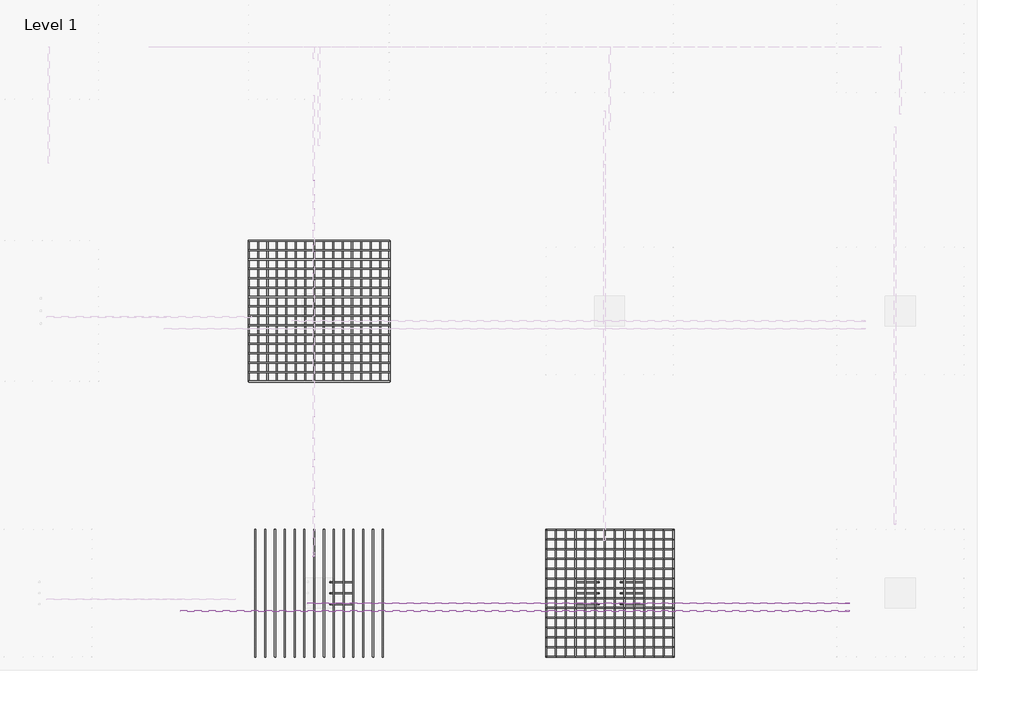
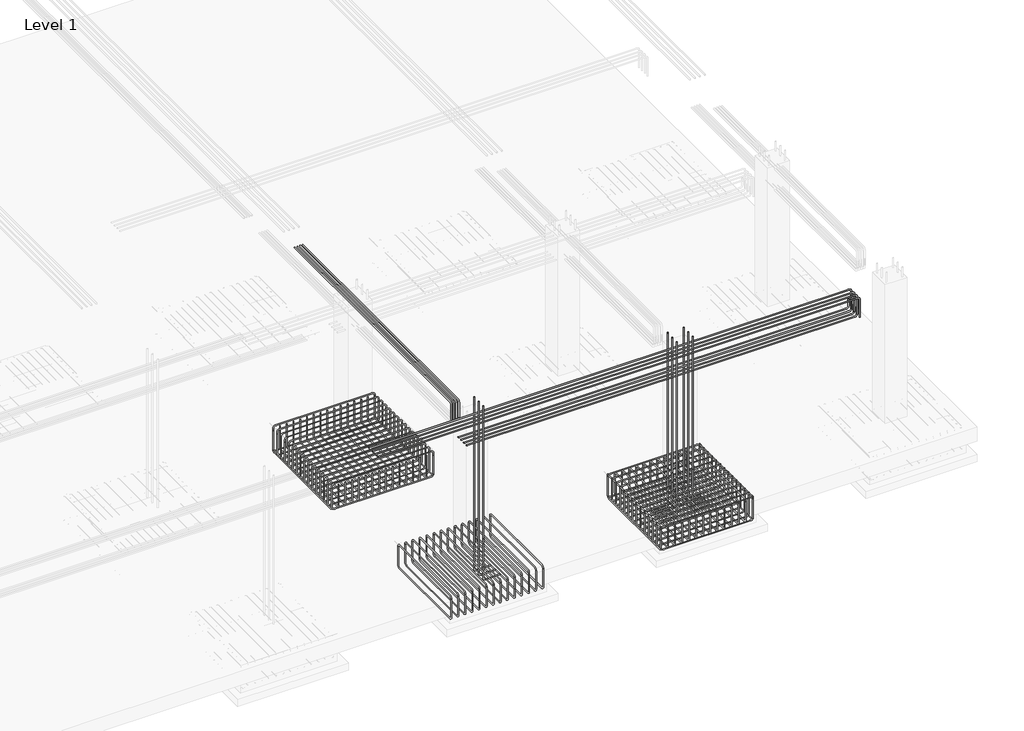
# One storey, part 6 of 17: 18 reinforcing bars.
"""IFC4 building model written with IfcOpenShell, lengths in millimetres."""

from ifc_helpers import new_model, si_unit, point, frame, origin, place, context, project, spatial, polyline, circle_curve, trimmed, segment, composite_curve, source, transform, mapped, element, save
from ifc_brep_helpers import swept_disk

model = new_model("IFC4")

# Units and contexts
model_context = context("Model", 3, world=origin())
ifc_project = project(units=[si_unit("LENGTHUNIT", "METRE", prefix="MILLI")], contexts=[model_context])

# Site, building, storey
site = spatial("IfcSite", under=ifc_project)
building = spatial("IfcBuilding", under=site)
storey = spatial("IfcBuildingStorey", under=building, Name="Level 1", Elevation=0.0)

# Reinforcing bars
placement = place(None, origin())
reinforcing_bar_shape = source(origin(), model_context, "Body", "SolidModel", [
    swept_disk(composite_curve([segment(polyline([(1252.6367997, -3580.990543, -96.0), (1252.6367997, -3580.990543, -504.0)]), True, "CONTINUOUS"), segment(trimmed(circle_curve(frame((1252.6367997, -3628.990543, -504.0), z_axis=(-1.0, 0.0, 0.0), x_axis=(0.0, 48.0, 0.0)), 48.0), [point((1252.6367997, -3580.990543, -504.0))], [point((1252.6367997, -3628.990543, -552.0))], True, "CARTESIAN"), True, "CONTINUOUS"), segment(polyline([(1252.6367997, -3628.990543, -552.0), (1252.6367997, -5436.990543, -552.0)]), True, "CONTINUOUS"), segment(trimmed(circle_curve(frame((1252.6367997, -5436.990543, -504.0), z_axis=(-1.0, 0.0, 0.0), x_axis=(0.0, 0.0, -48.0)), 48.0), [point((1252.6367997, -5436.990543, -552.0))], [point((1252.6367997, -5484.990543, -504.0))], True, "CARTESIAN"), True, "CONTINUOUS"), segment(polyline([(1252.6367997, -5484.990543, -504.0), (1252.6367997, -5484.990543, -96.0)]), True, "CONTINUOUS")], self_intersect=False), 8.0),
])
element("IfcReinforcingBar", 1, at=placement, inside=storey, context=model_context, shape_type="MappedRepresentation", body=[
    mapped(reinforcing_bar_shape, transform((0.0, 0.0, 0.0), x_axis=(1.0, 0.0, 0.0), y_axis=(0.0, 1.0, 0.0), z_axis=(0.0, 0.0, 1.0))),
    mapped(reinforcing_bar_shape, transform((-146.4615385, 0.0, 0.0), x_axis=(1.0, 0.0, 0.0), y_axis=(0.0, 1.0, 0.0), z_axis=(0.0, 0.0, 1.0))),
    mapped(reinforcing_bar_shape, transform((-292.9230769, 0.0, 0.0), x_axis=(1.0, 0.0, 0.0), y_axis=(0.0, 1.0, 0.0), z_axis=(0.0, 0.0, 1.0))),
    mapped(reinforcing_bar_shape, transform((-439.3846154, 0.0, 0.0), x_axis=(1.0, 0.0, 0.0), y_axis=(0.0, 1.0, 0.0), z_axis=(0.0, 0.0, 1.0))),
    mapped(reinforcing_bar_shape, transform((-585.8461538, 0.0, 0.0), x_axis=(1.0, 0.0, 0.0), y_axis=(0.0, 1.0, 0.0), z_axis=(0.0, 0.0, 1.0))),
    mapped(reinforcing_bar_shape, transform((-732.3076923, 0.0, 0.0), x_axis=(1.0, 0.0, 0.0), y_axis=(0.0, 1.0, 0.0), z_axis=(0.0, 0.0, 1.0))),
    mapped(reinforcing_bar_shape, transform((-878.7692308, 0.0, 0.0), x_axis=(1.0, 0.0, 0.0), y_axis=(0.0, 1.0, 0.0), z_axis=(0.0, 0.0, 1.0))),
    mapped(reinforcing_bar_shape, transform((-1025.2307692, 0.0, 0.0), x_axis=(1.0, 0.0, 0.0), y_axis=(0.0, 1.0, 0.0), z_axis=(0.0, 0.0, 1.0))),
    mapped(reinforcing_bar_shape, transform((-1171.6923077, 0.0, 0.0), x_axis=(1.0, 0.0, 0.0), y_axis=(0.0, 1.0, 0.0), z_axis=(0.0, 0.0, 1.0))),
    mapped(reinforcing_bar_shape, transform((-1318.1538462, 0.0, 0.0), x_axis=(1.0, 0.0, 0.0), y_axis=(0.0, 1.0, 0.0), z_axis=(0.0, 0.0, 1.0))),
    mapped(reinforcing_bar_shape, transform((-1464.6153846, 0.0, 0.0), x_axis=(1.0, 0.0, 0.0), y_axis=(0.0, 1.0, 0.0), z_axis=(0.0, 0.0, 1.0))),
    mapped(reinforcing_bar_shape, transform((-1611.0769231, 0.0, 0.0), x_axis=(1.0, 0.0, 0.0), y_axis=(0.0, 1.0, 0.0), z_axis=(0.0, 0.0, 1.0))),
    mapped(reinforcing_bar_shape, transform((-1757.5384615, 0.0, 0.0), x_axis=(1.0, 0.0, 0.0), y_axis=(0.0, 1.0, 0.0), z_axis=(0.0, 0.0, 1.0))),
    mapped(reinforcing_bar_shape, transform((-1904.0, 0.0, 0.0), x_axis=(1.0, 0.0, 0.0), y_axis=(0.0, 1.0, 0.0), z_axis=(0.0, 0.0, 1.0))),
])
reinforcing_bar_2_shape = source(origin(), model_context, "Body", "SolidModel", [
    swept_disk(composite_curve([segment(polyline([(-651.3632003, -3580.990543, -504.0), (-651.3632003, -3580.990543, -96.0)]), True, "CONTINUOUS"), segment(trimmed(circle_curve(frame((-651.3632003, -3628.990543, -96.0), z_axis=(1.0, 0.0, 0.0), x_axis=(0.0, 48.0, 0.0)), 48.0), [point((-651.3632003, -3580.990543, -96.0))], [point((-651.3632003, -3628.990543, -48.0))], True, "CARTESIAN"), True, "CONTINUOUS"), segment(polyline([(-651.3632003, -3628.990543, -48.0), (-651.3632003, -5436.990543, -48.0)]), True, "CONTINUOUS"), segment(trimmed(circle_curve(frame((-651.3632003, -5436.990543, -96.0), z_axis=(1.0, 0.0, 0.0), x_axis=(0.0, 0.0, 48.0)), 48.0), [point((-651.3632003, -5436.990543, -48.0))], [point((-651.3632003, -5484.990543, -96.0))], True, "CARTESIAN"), True, "CONTINUOUS"), segment(polyline([(-651.3632003, -5484.990543, -96.0), (-651.3632003, -5484.990543, -504.0)]), True, "CONTINUOUS")], self_intersect=False), 8.0),
])
element("IfcReinforcingBar", 2, at=placement, inside=storey, context=model_context, shape_type="MappedRepresentation", body=[
    mapped(reinforcing_bar_2_shape, transform((0.0, 0.0, 0.0), x_axis=(1.0, 0.0, 0.0), y_axis=(0.0, 1.0, 0.0), z_axis=(0.0, 0.0, 1.0))),
    mapped(reinforcing_bar_2_shape, transform((146.4615385, 0.0, 0.0), x_axis=(1.0, 0.0, 0.0), y_axis=(0.0, 1.0, 0.0), z_axis=(0.0, 0.0, 1.0))),
    mapped(reinforcing_bar_2_shape, transform((292.9230769, 0.0, 0.0), x_axis=(1.0, 0.0, 0.0), y_axis=(0.0, 1.0, 0.0), z_axis=(0.0, 0.0, 1.0))),
    mapped(reinforcing_bar_2_shape, transform((439.3846154, 0.0, 0.0), x_axis=(1.0, 0.0, 0.0), y_axis=(0.0, 1.0, 0.0), z_axis=(0.0, 0.0, 1.0))),
    mapped(reinforcing_bar_2_shape, transform((585.8461538, 0.0, 0.0), x_axis=(1.0, 0.0, 0.0), y_axis=(0.0, 1.0, 0.0), z_axis=(0.0, 0.0, 1.0))),
    mapped(reinforcing_bar_2_shape, transform((732.3076923, 0.0, 0.0), x_axis=(1.0, 0.0, 0.0), y_axis=(0.0, 1.0, 0.0), z_axis=(0.0, 0.0, 1.0))),
    mapped(reinforcing_bar_2_shape, transform((878.7692308, 0.0, 0.0), x_axis=(1.0, 0.0, 0.0), y_axis=(0.0, 1.0, 0.0), z_axis=(0.0, 0.0, 1.0))),
    mapped(reinforcing_bar_2_shape, transform((1025.2307692, 0.0, 0.0), x_axis=(1.0, 0.0, 0.0), y_axis=(0.0, 1.0, 0.0), z_axis=(0.0, 0.0, 1.0))),
    mapped(reinforcing_bar_2_shape, transform((1171.6923077, 0.0, 0.0), x_axis=(1.0, 0.0, 0.0), y_axis=(0.0, 1.0, 0.0), z_axis=(0.0, 0.0, 1.0))),
    mapped(reinforcing_bar_2_shape, transform((1318.1538462, 0.0, 0.0), x_axis=(1.0, 0.0, 0.0), y_axis=(0.0, 1.0, 0.0), z_axis=(0.0, 0.0, 1.0))),
    mapped(reinforcing_bar_2_shape, transform((1464.6153846, 0.0, 0.0), x_axis=(1.0, 0.0, 0.0), y_axis=(0.0, 1.0, 0.0), z_axis=(0.0, 0.0, 1.0))),
    mapped(reinforcing_bar_2_shape, transform((1611.0769231, 0.0, 0.0), x_axis=(1.0, 0.0, 0.0), y_axis=(0.0, 1.0, 0.0), z_axis=(0.0, 0.0, 1.0))),
    mapped(reinforcing_bar_2_shape, transform((1757.5384615, 0.0, 0.0), x_axis=(1.0, 0.0, 0.0), y_axis=(0.0, 1.0, 0.0), z_axis=(0.0, 0.0, 1.0))),
    mapped(reinforcing_bar_2_shape, transform((1904.0, 0.0, 0.0), x_axis=(1.0, 0.0, 0.0), y_axis=(0.0, 1.0, 0.0), z_axis=(0.0, 0.0, 1.0))),
])
reinforcing_bar_3_shape = source(origin(), model_context, "Body", "SolidModel", [
    swept_disk(composite_curve([segment(polyline([(813.2521843, -4698.490543, -550.0), (516.1367997, -4698.490543, -550.0)]), True, "CONTINUOUS"), segment(trimmed(circle_curve(frame((516.1367997, -4698.490543, -500.0), z_axis=(0.0, 1.0, 0.0), x_axis=(0.0, 0.0, -50.0)), 50.0), [point((516.1367997, -4698.490543, -550.0))], [point((466.1367997, -4698.490543, -500.0))], True, "CARTESIAN"), True, "CONTINUOUS"), segment(polyline([(466.1367997, -4698.490543, -500.0), (466.1367997, -4698.490543, 3260.0)]), True, "CONTINUOUS")], self_intersect=False), 10.0),
])
element("IfcReinforcingBar", 3, at=placement, inside=storey, context=model_context, shape_type="MappedRepresentation", body=[
    mapped(reinforcing_bar_3_shape, transform((0.0, 0.0, 0.0), x_axis=(1.0, 0.0, 0.0), y_axis=(0.0, 1.0, 0.0), z_axis=(0.0, 0.0, 1.0))),
    mapped(reinforcing_bar_3_shape, transform((0.0, 165.5, 0.0), x_axis=(1.0, 0.0, 0.0), y_axis=(0.0, 1.0, 0.0), z_axis=(0.0, 0.0, 1.0))),
    mapped(reinforcing_bar_3_shape, transform((0.0, 331.0, 0.0), x_axis=(1.0, 0.0, 0.0), y_axis=(0.0, 1.0, 0.0), z_axis=(0.0, 0.0, 1.0))),
])
reinforcing_bar_4_shape = source(origin(), model_context, "Body", "SolidModel", [
    swept_disk(composite_curve([segment(polyline([(3693.6367997, -3580.990543, -40.0), (3693.6367997, -3580.990543, -504.0)]), True, "CONTINUOUS"), segment(trimmed(circle_curve(frame((3741.6367997, -3580.990543, -504.0), z_axis=(0.0, -1.0, 0.0), x_axis=(-48.0, 0.0, 0.0)), 48.0), [point((3693.6367997, -3580.990543, -504.0))], [point((3741.6367997, -3580.990543, -552.0))], True, "CARTESIAN"), True, "CONTINUOUS"), segment(polyline([(3741.6367997, -3580.990543, -552.0), (5549.6367997, -3580.990543, -552.0)]), True, "CONTINUOUS"), segment(trimmed(circle_curve(frame((5549.6367997, -3580.990543, -504.0), z_axis=(0.0, -1.0, 0.0), x_axis=(0.0, 0.0, -48.0)), 48.0), [point((5549.6367997, -3580.990543, -552.0))], [point((5597.6367997, -3580.990543, -504.0))], True, "CARTESIAN"), True, "CONTINUOUS"), segment(polyline([(5597.6367997, -3580.990543, -504.0), (5597.6367997, -3580.990543, -40.0)]), True, "CONTINUOUS")], self_intersect=False), 8.0),
])
element("IfcReinforcingBar", 4, at=placement, inside=storey, context=model_context, shape_type="MappedRepresentation", body=[
    mapped(reinforcing_bar_4_shape, transform((0.0, 0.0, 0.0), x_axis=(1.0, 0.0, 0.0), y_axis=(0.0, 1.0, 0.0), z_axis=(0.0, 0.0, 1.0))),
    mapped(reinforcing_bar_4_shape, transform((0.0, -146.4615385, 0.0), x_axis=(1.0, 0.0, 0.0), y_axis=(0.0, 1.0, 0.0), z_axis=(0.0, 0.0, 1.0))),
    mapped(reinforcing_bar_4_shape, transform((0.0, -292.9230769, 0.0), x_axis=(1.0, 0.0, 0.0), y_axis=(0.0, 1.0, 0.0), z_axis=(0.0, 0.0, 1.0))),
    mapped(reinforcing_bar_4_shape, transform((0.0, -439.3846154, 0.0), x_axis=(1.0, 0.0, 0.0), y_axis=(0.0, 1.0, 0.0), z_axis=(0.0, 0.0, 1.0))),
    mapped(reinforcing_bar_4_shape, transform((0.0, -585.8461538, 0.0), x_axis=(1.0, 0.0, 0.0), y_axis=(0.0, 1.0, 0.0), z_axis=(0.0, 0.0, 1.0))),
    mapped(reinforcing_bar_4_shape, transform((0.0, -732.3076923, 0.0), x_axis=(1.0, 0.0, 0.0), y_axis=(0.0, 1.0, 0.0), z_axis=(0.0, 0.0, 1.0))),
    mapped(reinforcing_bar_4_shape, transform((0.0, -878.7692308, 0.0), x_axis=(1.0, 0.0, 0.0), y_axis=(0.0, 1.0, 0.0), z_axis=(0.0, 0.0, 1.0))),
    mapped(reinforcing_bar_4_shape, transform((0.0, -1025.2307692, 0.0), x_axis=(1.0, 0.0, 0.0), y_axis=(0.0, 1.0, 0.0), z_axis=(0.0, 0.0, 1.0))),
    mapped(reinforcing_bar_4_shape, transform((0.0, -1171.6923077, 0.0), x_axis=(1.0, 0.0, 0.0), y_axis=(0.0, 1.0, 0.0), z_axis=(0.0, 0.0, 1.0))),
    mapped(reinforcing_bar_4_shape, transform((0.0, -1318.1538462, 0.0), x_axis=(1.0, 0.0, 0.0), y_axis=(0.0, 1.0, 0.0), z_axis=(0.0, 0.0, 1.0))),
    mapped(reinforcing_bar_4_shape, transform((0.0, -1464.6153846, 0.0), x_axis=(1.0, 0.0, 0.0), y_axis=(0.0, 1.0, 0.0), z_axis=(0.0, 0.0, 1.0))),
    mapped(reinforcing_bar_4_shape, transform((0.0, -1611.0769231, 0.0), x_axis=(1.0, 0.0, 0.0), y_axis=(0.0, 1.0, 0.0), z_axis=(0.0, 0.0, 1.0))),
    mapped(reinforcing_bar_4_shape, transform((0.0, -1757.5384615, 0.0), x_axis=(1.0, 0.0, 0.0), y_axis=(0.0, 1.0, 0.0), z_axis=(0.0, 0.0, 1.0))),
    mapped(reinforcing_bar_4_shape, transform((0.0, -1904.0, 0.0), x_axis=(1.0, 0.0, 0.0), y_axis=(0.0, 1.0, 0.0), z_axis=(0.0, 0.0, 1.0))),
])
reinforcing_bar_5_shape = source(origin(), model_context, "Body", "SolidModel", [
    swept_disk(composite_curve([segment(polyline([(3693.6367997, -5484.990543, -504.0), (3693.6367997, -5484.990543, -96.0)]), True, "CONTINUOUS"), segment(trimmed(circle_curve(frame((3741.6367997, -5484.990543, -96.0), z_axis=(0.0, 1.0, 0.0), x_axis=(-48.0, 0.0, 0.0)), 48.0), [point((3693.6367997, -5484.990543, -96.0))], [point((3741.6367997, -5484.990543, -48.0))], True, "CARTESIAN"), True, "CONTINUOUS"), segment(polyline([(3741.6367997, -5484.990543, -48.0), (5549.6367997, -5484.990543, -48.0)]), True, "CONTINUOUS"), segment(trimmed(circle_curve(frame((5549.6367997, -5484.990543, -96.0), z_axis=(0.0, 1.0, 0.0), x_axis=(0.0, 0.0, 48.0)), 48.0), [point((5549.6367997, -5484.990543, -48.0))], [point((5597.6367997, -5484.990543, -96.0))], True, "CARTESIAN"), True, "CONTINUOUS"), segment(polyline([(5597.6367997, -5484.990543, -96.0), (5597.6367997, -5484.990543, -504.0)]), True, "CONTINUOUS")], self_intersect=False), 8.0),
])
element("IfcReinforcingBar", 5, at=placement, inside=storey, context=model_context, shape_type="MappedRepresentation", body=[
    mapped(reinforcing_bar_5_shape, transform((0.0, 0.0, 0.0), x_axis=(1.0, 0.0, 0.0), y_axis=(0.0, 1.0, 0.0), z_axis=(0.0, 0.0, 1.0))),
    mapped(reinforcing_bar_5_shape, transform((0.0, 146.4615385, 0.0), x_axis=(1.0, 0.0, 0.0), y_axis=(0.0, 1.0, 0.0), z_axis=(0.0, 0.0, 1.0))),
    mapped(reinforcing_bar_5_shape, transform((0.0, 292.9230769, 0.0), x_axis=(1.0, 0.0, 0.0), y_axis=(0.0, 1.0, 0.0), z_axis=(0.0, 0.0, 1.0))),
    mapped(reinforcing_bar_5_shape, transform((0.0, 439.3846154, 0.0), x_axis=(1.0, 0.0, 0.0), y_axis=(0.0, 1.0, 0.0), z_axis=(0.0, 0.0, 1.0))),
    mapped(reinforcing_bar_5_shape, transform((0.0, 585.8461538, 0.0), x_axis=(1.0, 0.0, 0.0), y_axis=(0.0, 1.0, 0.0), z_axis=(0.0, 0.0, 1.0))),
    mapped(reinforcing_bar_5_shape, transform((0.0, 732.3076923, 0.0), x_axis=(1.0, 0.0, 0.0), y_axis=(0.0, 1.0, 0.0), z_axis=(0.0, 0.0, 1.0))),
    mapped(reinforcing_bar_5_shape, transform((0.0, 878.7692308, 0.0), x_axis=(1.0, 0.0, 0.0), y_axis=(0.0, 1.0, 0.0), z_axis=(0.0, 0.0, 1.0))),
    mapped(reinforcing_bar_5_shape, transform((0.0, 1025.2307692, 0.0), x_axis=(1.0, 0.0, 0.0), y_axis=(0.0, 1.0, 0.0), z_axis=(0.0, 0.0, 1.0))),
    mapped(reinforcing_bar_5_shape, transform((0.0, 1171.6923077, 0.0), x_axis=(1.0, 0.0, 0.0), y_axis=(0.0, 1.0, 0.0), z_axis=(0.0, 0.0, 1.0))),
    mapped(reinforcing_bar_5_shape, transform((0.0, 1318.1538462, 0.0), x_axis=(1.0, 0.0, 0.0), y_axis=(0.0, 1.0, 0.0), z_axis=(0.0, 0.0, 1.0))),
    mapped(reinforcing_bar_5_shape, transform((0.0, 1464.6153846, 0.0), x_axis=(1.0, 0.0, 0.0), y_axis=(0.0, 1.0, 0.0), z_axis=(0.0, 0.0, 1.0))),
    mapped(reinforcing_bar_5_shape, transform((0.0, 1611.0769231, 0.0), x_axis=(1.0, 0.0, 0.0), y_axis=(0.0, 1.0, 0.0), z_axis=(0.0, 0.0, 1.0))),
    mapped(reinforcing_bar_5_shape, transform((0.0, 1757.5384615, 0.0), x_axis=(1.0, 0.0, 0.0), y_axis=(0.0, 1.0, 0.0), z_axis=(0.0, 0.0, 1.0))),
    mapped(reinforcing_bar_5_shape, transform((0.0, 1904.0, 0.0), x_axis=(1.0, 0.0, 0.0), y_axis=(0.0, 1.0, 0.0), z_axis=(0.0, 0.0, 1.0))),
])
reinforcing_bar_6_shape = source(origin(), model_context, "Body", "SolidModel", [
    swept_disk(composite_curve([segment(polyline([(5597.6367997, -3580.990543, -96.0), (5597.6367997, -3580.990543, -504.0)]), True, "CONTINUOUS"), segment(trimmed(circle_curve(frame((5597.6367997, -3628.990543, -504.0), z_axis=(-1.0, 0.0, 0.0), x_axis=(0.0, 48.0, 0.0)), 48.0), [point((5597.6367997, -3580.990543, -504.0))], [point((5597.6367997, -3628.990543, -552.0))], True, "CARTESIAN"), True, "CONTINUOUS"), segment(polyline([(5597.6367997, -3628.990543, -552.0), (5597.6367997, -5436.990543, -552.0)]), True, "CONTINUOUS"), segment(trimmed(circle_curve(frame((5597.6367997, -5436.990543, -504.0), z_axis=(-1.0, 0.0, 0.0), x_axis=(0.0, 0.0, -48.0)), 48.0), [point((5597.6367997, -5436.990543, -552.0))], [point((5597.6367997, -5484.990543, -504.0))], True, "CARTESIAN"), True, "CONTINUOUS"), segment(polyline([(5597.6367997, -5484.990543, -504.0), (5597.6367997, -5484.990543, -96.0)]), True, "CONTINUOUS")], self_intersect=False), 8.0),
])
element("IfcReinforcingBar", 6, at=placement, inside=storey, context=model_context, shape_type="MappedRepresentation", body=[
    mapped(reinforcing_bar_6_shape, transform((0.0, 0.0, 0.0), x_axis=(1.0, 0.0, 0.0), y_axis=(0.0, 1.0, 0.0), z_axis=(0.0, 0.0, 1.0))),
    mapped(reinforcing_bar_6_shape, transform((-146.4615385, 0.0, 0.0), x_axis=(1.0, 0.0, 0.0), y_axis=(0.0, 1.0, 0.0), z_axis=(0.0, 0.0, 1.0))),
    mapped(reinforcing_bar_6_shape, transform((-292.9230769, 0.0, 0.0), x_axis=(1.0, 0.0, 0.0), y_axis=(0.0, 1.0, 0.0), z_axis=(0.0, 0.0, 1.0))),
    mapped(reinforcing_bar_6_shape, transform((-439.3846154, 0.0, 0.0), x_axis=(1.0, 0.0, 0.0), y_axis=(0.0, 1.0, 0.0), z_axis=(0.0, 0.0, 1.0))),
    mapped(reinforcing_bar_6_shape, transform((-585.8461538, 0.0, 0.0), x_axis=(1.0, 0.0, 0.0), y_axis=(0.0, 1.0, 0.0), z_axis=(0.0, 0.0, 1.0))),
    mapped(reinforcing_bar_6_shape, transform((-732.3076923, 0.0, 0.0), x_axis=(1.0, 0.0, 0.0), y_axis=(0.0, 1.0, 0.0), z_axis=(0.0, 0.0, 1.0))),
    mapped(reinforcing_bar_6_shape, transform((-878.7692308, 0.0, 0.0), x_axis=(1.0, 0.0, 0.0), y_axis=(0.0, 1.0, 0.0), z_axis=(0.0, 0.0, 1.0))),
    mapped(reinforcing_bar_6_shape, transform((-1025.2307692, 0.0, 0.0), x_axis=(1.0, 0.0, 0.0), y_axis=(0.0, 1.0, 0.0), z_axis=(0.0, 0.0, 1.0))),
    mapped(reinforcing_bar_6_shape, transform((-1171.6923077, 0.0, 0.0), x_axis=(1.0, 0.0, 0.0), y_axis=(0.0, 1.0, 0.0), z_axis=(0.0, 0.0, 1.0))),
    mapped(reinforcing_bar_6_shape, transform((-1318.1538462, 0.0, 0.0), x_axis=(1.0, 0.0, 0.0), y_axis=(0.0, 1.0, 0.0), z_axis=(0.0, 0.0, 1.0))),
    mapped(reinforcing_bar_6_shape, transform((-1464.6153846, 0.0, 0.0), x_axis=(1.0, 0.0, 0.0), y_axis=(0.0, 1.0, 0.0), z_axis=(0.0, 0.0, 1.0))),
    mapped(reinforcing_bar_6_shape, transform((-1611.0769231, 0.0, 0.0), x_axis=(1.0, 0.0, 0.0), y_axis=(0.0, 1.0, 0.0), z_axis=(0.0, 0.0, 1.0))),
    mapped(reinforcing_bar_6_shape, transform((-1757.5384615, 0.0, 0.0), x_axis=(1.0, 0.0, 0.0), y_axis=(0.0, 1.0, 0.0), z_axis=(0.0, 0.0, 1.0))),
    mapped(reinforcing_bar_6_shape, transform((-1904.0, 0.0, 0.0), x_axis=(1.0, 0.0, 0.0), y_axis=(0.0, 1.0, 0.0), z_axis=(0.0, 0.0, 1.0))),
])
reinforcing_bar_7_shape = source(origin(), model_context, "Body", "SolidModel", [
    swept_disk(composite_curve([segment(polyline([(3693.6367997, -3580.990543, -504.0), (3693.6367997, -3580.990543, -96.0)]), True, "CONTINUOUS"), segment(trimmed(circle_curve(frame((3693.6367997, -3628.990543, -96.0), z_axis=(1.0, 0.0, 0.0), x_axis=(0.0, 48.0, 0.0)), 48.0), [point((3693.6367997, -3580.990543, -96.0))], [point((3693.6367997, -3628.990543, -48.0))], True, "CARTESIAN"), True, "CONTINUOUS"), segment(polyline([(3693.6367997, -3628.990543, -48.0), (3693.6367997, -5436.990543, -48.0)]), True, "CONTINUOUS"), segment(trimmed(circle_curve(frame((3693.6367997, -5436.990543, -96.0), z_axis=(1.0, 0.0, 0.0), x_axis=(0.0, 0.0, 48.0)), 48.0), [point((3693.6367997, -5436.990543, -48.0))], [point((3693.6367997, -5484.990543, -96.0))], True, "CARTESIAN"), True, "CONTINUOUS"), segment(polyline([(3693.6367997, -5484.990543, -96.0), (3693.6367997, -5484.990543, -504.0)]), True, "CONTINUOUS")], self_intersect=False), 8.0),
])
element("IfcReinforcingBar", 7, at=placement, inside=storey, context=model_context, shape_type="MappedRepresentation", body=[
    mapped(reinforcing_bar_7_shape, transform((0.0, 0.0, 0.0), x_axis=(1.0, 0.0, 0.0), y_axis=(0.0, 1.0, 0.0), z_axis=(0.0, 0.0, 1.0))),
    mapped(reinforcing_bar_7_shape, transform((146.4615385, 0.0, 0.0), x_axis=(1.0, 0.0, 0.0), y_axis=(0.0, 1.0, 0.0), z_axis=(0.0, 0.0, 1.0))),
    mapped(reinforcing_bar_7_shape, transform((292.9230769, 0.0, 0.0), x_axis=(1.0, 0.0, 0.0), y_axis=(0.0, 1.0, 0.0), z_axis=(0.0, 0.0, 1.0))),
    mapped(reinforcing_bar_7_shape, transform((439.3846154, 0.0, 0.0), x_axis=(1.0, 0.0, 0.0), y_axis=(0.0, 1.0, 0.0), z_axis=(0.0, 0.0, 1.0))),
    mapped(reinforcing_bar_7_shape, transform((585.8461538, 0.0, 0.0), x_axis=(1.0, 0.0, 0.0), y_axis=(0.0, 1.0, 0.0), z_axis=(0.0, 0.0, 1.0))),
    mapped(reinforcing_bar_7_shape, transform((732.3076923, 0.0, 0.0), x_axis=(1.0, 0.0, 0.0), y_axis=(0.0, 1.0, 0.0), z_axis=(0.0, 0.0, 1.0))),
    mapped(reinforcing_bar_7_shape, transform((878.7692308, 0.0, 0.0), x_axis=(1.0, 0.0, 0.0), y_axis=(0.0, 1.0, 0.0), z_axis=(0.0, 0.0, 1.0))),
    mapped(reinforcing_bar_7_shape, transform((1025.2307692, 0.0, 0.0), x_axis=(1.0, 0.0, 0.0), y_axis=(0.0, 1.0, 0.0), z_axis=(0.0, 0.0, 1.0))),
    mapped(reinforcing_bar_7_shape, transform((1171.6923077, 0.0, 0.0), x_axis=(1.0, 0.0, 0.0), y_axis=(0.0, 1.0, 0.0), z_axis=(0.0, 0.0, 1.0))),
    mapped(reinforcing_bar_7_shape, transform((1318.1538462, 0.0, 0.0), x_axis=(1.0, 0.0, 0.0), y_axis=(0.0, 1.0, 0.0), z_axis=(0.0, 0.0, 1.0))),
    mapped(reinforcing_bar_7_shape, transform((1464.6153846, 0.0, 0.0), x_axis=(1.0, 0.0, 0.0), y_axis=(0.0, 1.0, 0.0), z_axis=(0.0, 0.0, 1.0))),
    mapped(reinforcing_bar_7_shape, transform((1611.0769231, 0.0, 0.0), x_axis=(1.0, 0.0, 0.0), y_axis=(0.0, 1.0, 0.0), z_axis=(0.0, 0.0, 1.0))),
    mapped(reinforcing_bar_7_shape, transform((1757.5384615, 0.0, 0.0), x_axis=(1.0, 0.0, 0.0), y_axis=(0.0, 1.0, 0.0), z_axis=(0.0, 0.0, 1.0))),
    mapped(reinforcing_bar_7_shape, transform((1904.0, 0.0, 0.0), x_axis=(1.0, 0.0, 0.0), y_axis=(0.0, 1.0, 0.0), z_axis=(0.0, 0.0, 1.0))),
])
reinforcing_bar_8_shape = source(origin(), model_context, "Body", "SolidModel", [
    swept_disk(composite_curve([segment(polyline([(4133.0214151, -4367.490543, -550.0), (4430.1367997, -4367.490543, -550.0)]), True, "CONTINUOUS"), segment(trimmed(circle_curve(frame((4430.1367997, -4367.490543, -500.0), z_axis=(0.0, -1.0, 0.0), x_axis=(0.0, 0.0, -50.0)), 50.0), [point((4430.1367997, -4367.490543, -550.0))], [point((4480.1367997, -4367.490543, -500.0))], True, "CARTESIAN"), True, "CONTINUOUS"), segment(polyline([(4480.1367997, -4367.490543, -500.0), (4480.1367997, -4367.490543, 3260.0)]), True, "CONTINUOUS")], self_intersect=False), 10.0),
])
element("IfcReinforcingBar", 8, at=placement, inside=storey, context=model_context, shape_type="MappedRepresentation", body=[
    mapped(reinforcing_bar_8_shape, transform((0.0, 0.0, 0.0), x_axis=(1.0, 0.0, 0.0), y_axis=(0.0, 1.0, 0.0), z_axis=(0.0, 0.0, 1.0))),
    mapped(reinforcing_bar_8_shape, transform((0.0, -165.5, 0.0), x_axis=(1.0, 0.0, 0.0), y_axis=(0.0, 1.0, 0.0), z_axis=(0.0, 0.0, 1.0))),
    mapped(reinforcing_bar_8_shape, transform((0.0, -331.0, 0.0), x_axis=(1.0, 0.0, 0.0), y_axis=(0.0, 1.0, 0.0), z_axis=(0.0, 0.0, 1.0))),
])
reinforcing_bar_9_shape = source(origin(), model_context, "Body", "SolidModel", [
    swept_disk(composite_curve([segment(polyline([(5158.2521843, -4698.490543, -550.0), (4861.1367997, -4698.490543, -550.0)]), True, "CONTINUOUS"), segment(trimmed(circle_curve(frame((4861.1367997, -4698.490543, -500.0), z_axis=(0.0, 1.0, 0.0), x_axis=(0.0, 0.0, -50.0)), 50.0), [point((4861.1367997, -4698.490543, -550.0))], [point((4811.1367997, -4698.490543, -500.0))], True, "CARTESIAN"), True, "CONTINUOUS"), segment(polyline([(4811.1367997, -4698.490543, -500.0), (4811.1367997, -4698.490543, 3260.0)]), True, "CONTINUOUS")], self_intersect=False), 10.0),
])
element("IfcReinforcingBar", 9, at=placement, inside=storey, context=model_context, shape_type="MappedRepresentation", body=[
    mapped(reinforcing_bar_9_shape, transform((0.0, 0.0, 0.0), x_axis=(1.0, 0.0, 0.0), y_axis=(0.0, 1.0, 0.0), z_axis=(0.0, 0.0, 1.0))),
    mapped(reinforcing_bar_9_shape, transform((0.0, 165.5, 0.0), x_axis=(1.0, 0.0, 0.0), y_axis=(0.0, 1.0, 0.0), z_axis=(0.0, 0.0, 1.0))),
    mapped(reinforcing_bar_9_shape, transform((0.0, 331.0, 0.0), x_axis=(1.0, 0.0, 0.0), y_axis=(0.0, 1.0, 0.0), z_axis=(0.0, 0.0, 1.0))),
])
reinforcing_bar_10_shape = source(origin(), model_context, "Body", "SolidModel", [
    swept_disk(composite_curve([segment(polyline([(-751.3632003, 736.009457, -140.0), (-751.3632003, 736.009457, -554.0)]), True, "CONTINUOUS"), segment(trimmed(circle_curve(frame((-703.3632003, 736.009457, -554.0), z_axis=(0.0, -1.0, 0.0), x_axis=(-48.0, 0.0, 0.0)), 48.0), [point((-751.3632003, 736.009457, -554.0))], [point((-703.3632003, 736.009457, -602.0))], True, "CARTESIAN"), True, "CONTINUOUS"), segment(polyline([(-703.3632003, 736.009457, -602.0), (1304.6367997, 736.009457, -602.0)]), True, "CONTINUOUS"), segment(trimmed(circle_curve(frame((1304.6367997, 736.009457, -554.0), z_axis=(0.0, -1.0, 0.0), x_axis=(0.0, 0.0, -48.0)), 48.0), [point((1304.6367997, 736.009457, -602.0))], [point((1352.6367997, 736.009457, -554.0))], True, "CARTESIAN"), True, "CONTINUOUS"), segment(polyline([(1352.6367997, 736.009457, -554.0), (1352.6367997, 736.009457, -140.0)]), True, "CONTINUOUS")], self_intersect=False), 8.0),
])
element("IfcReinforcingBar", 10, at=placement, inside=storey, context=model_context, shape_type="MappedRepresentation", body=[
    mapped(reinforcing_bar_10_shape, transform((0.0, 0.0, 0.0), x_axis=(1.0, 0.0, 0.0), y_axis=(0.0, 1.0, 0.0), z_axis=(0.0, 0.0, 1.0))),
    mapped(reinforcing_bar_10_shape, transform((0.0, -140.2666667, 0.0), x_axis=(1.0, 0.0, 0.0), y_axis=(0.0, 1.0, 0.0), z_axis=(0.0, 0.0, 1.0))),
    mapped(reinforcing_bar_10_shape, transform((0.0, -280.5333333, 0.0), x_axis=(1.0, 0.0, 0.0), y_axis=(0.0, 1.0, 0.0), z_axis=(0.0, 0.0, 1.0))),
    mapped(reinforcing_bar_10_shape, transform((0.0, -420.8, 0.0), x_axis=(1.0, 0.0, 0.0), y_axis=(0.0, 1.0, 0.0), z_axis=(0.0, 0.0, 1.0))),
    mapped(reinforcing_bar_10_shape, transform((0.0, -561.0666667, 0.0), x_axis=(1.0, 0.0, 0.0), y_axis=(0.0, 1.0, 0.0), z_axis=(0.0, 0.0, 1.0))),
    mapped(reinforcing_bar_10_shape, transform((0.0, -701.3333333, 0.0), x_axis=(1.0, 0.0, 0.0), y_axis=(0.0, 1.0, 0.0), z_axis=(0.0, 0.0, 1.0))),
    mapped(reinforcing_bar_10_shape, transform((0.0, -841.6, 0.0), x_axis=(1.0, 0.0, 0.0), y_axis=(0.0, 1.0, 0.0), z_axis=(0.0, 0.0, 1.0))),
    mapped(reinforcing_bar_10_shape, transform((0.0, -981.8666667, 0.0), x_axis=(1.0, 0.0, 0.0), y_axis=(0.0, 1.0, 0.0), z_axis=(0.0, 0.0, 1.0))),
    mapped(reinforcing_bar_10_shape, transform((0.0, -1122.1333333, 0.0), x_axis=(1.0, 0.0, 0.0), y_axis=(0.0, 1.0, 0.0), z_axis=(0.0, 0.0, 1.0))),
    mapped(reinforcing_bar_10_shape, transform((0.0, -1262.4, 0.0), x_axis=(1.0, 0.0, 0.0), y_axis=(0.0, 1.0, 0.0), z_axis=(0.0, 0.0, 1.0))),
    mapped(reinforcing_bar_10_shape, transform((0.0, -1402.6666667, 0.0), x_axis=(1.0, 0.0, 0.0), y_axis=(0.0, 1.0, 0.0), z_axis=(0.0, 0.0, 1.0))),
    mapped(reinforcing_bar_10_shape, transform((0.0, -1542.9333333, 0.0), x_axis=(1.0, 0.0, 0.0), y_axis=(0.0, 1.0, 0.0), z_axis=(0.0, 0.0, 1.0))),
    mapped(reinforcing_bar_10_shape, transform((0.0, -1683.2, 0.0), x_axis=(1.0, 0.0, 0.0), y_axis=(0.0, 1.0, 0.0), z_axis=(0.0, 0.0, 1.0))),
    mapped(reinforcing_bar_10_shape, transform((0.0, -1823.4666667, 0.0), x_axis=(1.0, 0.0, 0.0), y_axis=(0.0, 1.0, 0.0), z_axis=(0.0, 0.0, 1.0))),
    mapped(reinforcing_bar_10_shape, transform((0.0, -1963.7333333, 0.0), x_axis=(1.0, 0.0, 0.0), y_axis=(0.0, 1.0, 0.0), z_axis=(0.0, 0.0, 1.0))),
    mapped(reinforcing_bar_10_shape, transform((0.0, -2104.0, 0.0), x_axis=(1.0, 0.0, 0.0), y_axis=(0.0, 1.0, 0.0), z_axis=(0.0, 0.0, 1.0))),
])
reinforcing_bar_11_shape = source(origin(), model_context, "Body", "SolidModel", [
    swept_disk(composite_curve([segment(polyline([(-751.3632003, -1367.990543, -554.0), (-751.3632003, -1367.990543, -96.0)]), True, "CONTINUOUS"), segment(trimmed(circle_curve(frame((-703.3632003, -1367.990543, -96.0), z_axis=(0.0, 1.0, 0.0), x_axis=(-48.0, 0.0, 0.0)), 48.0), [point((-751.3632003, -1367.990543, -96.0))], [point((-703.3632003, -1367.990543, -48.0))], True, "CARTESIAN"), True, "CONTINUOUS"), segment(polyline([(-703.3632003, -1367.990543, -48.0), (1304.6367997, -1367.990543, -48.0)]), True, "CONTINUOUS"), segment(trimmed(circle_curve(frame((1304.6367997, -1367.990543, -96.0), z_axis=(0.0, 1.0, 0.0), x_axis=(0.0, 0.0, 48.0)), 48.0), [point((1304.6367997, -1367.990543, -48.0))], [point((1352.6367997, -1367.990543, -96.0))], True, "CARTESIAN"), True, "CONTINUOUS"), segment(polyline([(1352.6367997, -1367.990543, -96.0), (1352.6367997, -1367.990543, -554.0)]), True, "CONTINUOUS")], self_intersect=False), 8.0),
])
element("IfcReinforcingBar", 11, at=placement, inside=storey, context=model_context, shape_type="MappedRepresentation", body=[
    mapped(reinforcing_bar_11_shape, transform((0.0, 0.0, 0.0), x_axis=(1.0, 0.0, 0.0), y_axis=(0.0, 1.0, 0.0), z_axis=(0.0, 0.0, 1.0))),
    mapped(reinforcing_bar_11_shape, transform((0.0, 140.2666667, 0.0), x_axis=(1.0, 0.0, 0.0), y_axis=(0.0, 1.0, 0.0), z_axis=(0.0, 0.0, 1.0))),
    mapped(reinforcing_bar_11_shape, transform((0.0, 280.5333333, 0.0), x_axis=(1.0, 0.0, 0.0), y_axis=(0.0, 1.0, 0.0), z_axis=(0.0, 0.0, 1.0))),
    mapped(reinforcing_bar_11_shape, transform((0.0, 420.8, 0.0), x_axis=(1.0, 0.0, 0.0), y_axis=(0.0, 1.0, 0.0), z_axis=(0.0, 0.0, 1.0))),
    mapped(reinforcing_bar_11_shape, transform((0.0, 561.0666667, 0.0), x_axis=(1.0, 0.0, 0.0), y_axis=(0.0, 1.0, 0.0), z_axis=(0.0, 0.0, 1.0))),
    mapped(reinforcing_bar_11_shape, transform((0.0, 701.3333333, 0.0), x_axis=(1.0, 0.0, 0.0), y_axis=(0.0, 1.0, 0.0), z_axis=(0.0, 0.0, 1.0))),
    mapped(reinforcing_bar_11_shape, transform((0.0, 841.6, 0.0), x_axis=(1.0, 0.0, 0.0), y_axis=(0.0, 1.0, 0.0), z_axis=(0.0, 0.0, 1.0))),
    mapped(reinforcing_bar_11_shape, transform((0.0, 981.8666667, 0.0), x_axis=(1.0, 0.0, 0.0), y_axis=(0.0, 1.0, 0.0), z_axis=(0.0, 0.0, 1.0))),
    mapped(reinforcing_bar_11_shape, transform((0.0, 1122.1333333, 0.0), x_axis=(1.0, 0.0, 0.0), y_axis=(0.0, 1.0, 0.0), z_axis=(0.0, 0.0, 1.0))),
    mapped(reinforcing_bar_11_shape, transform((0.0, 1262.4, 0.0), x_axis=(1.0, 0.0, 0.0), y_axis=(0.0, 1.0, 0.0), z_axis=(0.0, 0.0, 1.0))),
    mapped(reinforcing_bar_11_shape, transform((0.0, 1402.6666667, 0.0), x_axis=(1.0, 0.0, 0.0), y_axis=(0.0, 1.0, 0.0), z_axis=(0.0, 0.0, 1.0))),
    mapped(reinforcing_bar_11_shape, transform((0.0, 1542.9333333, 0.0), x_axis=(1.0, 0.0, 0.0), y_axis=(0.0, 1.0, 0.0), z_axis=(0.0, 0.0, 1.0))),
    mapped(reinforcing_bar_11_shape, transform((0.0, 1683.2, 0.0), x_axis=(1.0, 0.0, 0.0), y_axis=(0.0, 1.0, 0.0), z_axis=(0.0, 0.0, 1.0))),
    mapped(reinforcing_bar_11_shape, transform((0.0, 1823.4666667, 0.0), x_axis=(1.0, 0.0, 0.0), y_axis=(0.0, 1.0, 0.0), z_axis=(0.0, 0.0, 1.0))),
    mapped(reinforcing_bar_11_shape, transform((0.0, 1963.7333333, 0.0), x_axis=(1.0, 0.0, 0.0), y_axis=(0.0, 1.0, 0.0), z_axis=(0.0, 0.0, 1.0))),
    mapped(reinforcing_bar_11_shape, transform((0.0, 2104.0, 0.0), x_axis=(1.0, 0.0, 0.0), y_axis=(0.0, 1.0, 0.0), z_axis=(0.0, 0.0, 1.0))),
])
reinforcing_bar_12_shape = source(origin(), model_context, "Body", "SolidModel", [
    swept_disk(composite_curve([segment(polyline([(1352.6367997, 736.009457, -100.0), (1352.6367997, 736.009457, -554.0)]), True, "CONTINUOUS"), segment(trimmed(circle_curve(frame((1352.6367997, 688.009457, -554.0), z_axis=(-1.0, 0.0, 0.0), x_axis=(0.0, 48.0, 0.0)), 48.0), [point((1352.6367997, 736.009457, -554.0))], [point((1352.6367997, 688.009457, -602.0))], True, "CARTESIAN"), True, "CONTINUOUS"), segment(polyline([(1352.6367997, 688.009457, -602.0), (1352.6367997, -1319.990543, -602.0)]), True, "CONTINUOUS"), segment(trimmed(circle_curve(frame((1352.6367997, -1319.990543, -554.0), z_axis=(-1.0, 0.0, 0.0), x_axis=(0.0, 0.0, -48.0)), 48.0), [point((1352.6367997, -1319.990543, -602.0))], [point((1352.6367997, -1367.990543, -554.0))], True, "CARTESIAN"), True, "CONTINUOUS"), segment(polyline([(1352.6367997, -1367.990543, -554.0), (1352.6367997, -1367.990543, -100.0)]), True, "CONTINUOUS")], self_intersect=False), 8.0),
])
element("IfcReinforcingBar", 12, at=placement, inside=storey, context=model_context, shape_type="MappedRepresentation", body=[
    mapped(reinforcing_bar_12_shape, transform((0.0, 0.0, 0.0), x_axis=(1.0, 0.0, 0.0), y_axis=(0.0, 1.0, 0.0), z_axis=(0.0, 0.0, 1.0))),
    mapped(reinforcing_bar_12_shape, transform((-140.2666667, 0.0, 0.0), x_axis=(1.0, 0.0, 0.0), y_axis=(0.0, 1.0, 0.0), z_axis=(0.0, 0.0, 1.0))),
    mapped(reinforcing_bar_12_shape, transform((-280.5333333, 0.0, 0.0), x_axis=(1.0, 0.0, 0.0), y_axis=(0.0, 1.0, 0.0), z_axis=(0.0, 0.0, 1.0))),
    mapped(reinforcing_bar_12_shape, transform((-420.8, 0.0, 0.0), x_axis=(1.0, 0.0, 0.0), y_axis=(0.0, 1.0, 0.0), z_axis=(0.0, 0.0, 1.0))),
    mapped(reinforcing_bar_12_shape, transform((-561.0666667, 0.0, 0.0), x_axis=(1.0, 0.0, 0.0), y_axis=(0.0, 1.0, 0.0), z_axis=(0.0, 0.0, 1.0))),
    mapped(reinforcing_bar_12_shape, transform((-701.3333333, 0.0, 0.0), x_axis=(1.0, 0.0, 0.0), y_axis=(0.0, 1.0, 0.0), z_axis=(0.0, 0.0, 1.0))),
    mapped(reinforcing_bar_12_shape, transform((-841.6, 0.0, 0.0), x_axis=(1.0, 0.0, 0.0), y_axis=(0.0, 1.0, 0.0), z_axis=(0.0, 0.0, 1.0))),
    mapped(reinforcing_bar_12_shape, transform((-981.8666667, 0.0, 0.0), x_axis=(1.0, 0.0, 0.0), y_axis=(0.0, 1.0, 0.0), z_axis=(0.0, 0.0, 1.0))),
    mapped(reinforcing_bar_12_shape, transform((-1122.1333333, 0.0, 0.0), x_axis=(1.0, 0.0, 0.0), y_axis=(0.0, 1.0, 0.0), z_axis=(0.0, 0.0, 1.0))),
    mapped(reinforcing_bar_12_shape, transform((-1262.4, 0.0, 0.0), x_axis=(1.0, 0.0, 0.0), y_axis=(0.0, 1.0, 0.0), z_axis=(0.0, 0.0, 1.0))),
    mapped(reinforcing_bar_12_shape, transform((-1402.6666667, 0.0, 0.0), x_axis=(1.0, 0.0, 0.0), y_axis=(0.0, 1.0, 0.0), z_axis=(0.0, 0.0, 1.0))),
    mapped(reinforcing_bar_12_shape, transform((-1542.9333333, 0.0, 0.0), x_axis=(1.0, 0.0, 0.0), y_axis=(0.0, 1.0, 0.0), z_axis=(0.0, 0.0, 1.0))),
    mapped(reinforcing_bar_12_shape, transform((-1683.2, 0.0, 0.0), x_axis=(1.0, 0.0, 0.0), y_axis=(0.0, 1.0, 0.0), z_axis=(0.0, 0.0, 1.0))),
    mapped(reinforcing_bar_12_shape, transform((-1823.4666667, 0.0, 0.0), x_axis=(1.0, 0.0, 0.0), y_axis=(0.0, 1.0, 0.0), z_axis=(0.0, 0.0, 1.0))),
    mapped(reinforcing_bar_12_shape, transform((-1963.7333333, 0.0, 0.0), x_axis=(1.0, 0.0, 0.0), y_axis=(0.0, 1.0, 0.0), z_axis=(0.0, 0.0, 1.0))),
    mapped(reinforcing_bar_12_shape, transform((-2104.0, 0.0, 0.0), x_axis=(1.0, 0.0, 0.0), y_axis=(0.0, 1.0, 0.0), z_axis=(0.0, 0.0, 1.0))),
])
reinforcing_bar_13_shape = source(origin(), model_context, "Body", "SolidModel", [
    swept_disk(composite_curve([segment(polyline([(8214.8367997, -4683.490543, 2707.4), (8214.8367997, -4683.490543, 2557.5)]), True, "CONTINUOUS"), segment(trimmed(circle_curve(frame((8164.8367997, -4683.490543, 2557.5), z_axis=(0.0, 1.0, 0.0), x_axis=(50.00000000000091, 0.0, 0.0)), 50.0), [point((8214.8367997, -4683.490543, 2557.5))], [point((8164.8367997, -4683.490543, 2507.5))], True, "CARTESIAN"), True, "CONTINUOUS"), segment(polyline([(8164.8367997, -4683.490543, 2507.5), (126.4367997, -4683.490543, 2507.5)]), True, "CONTINUOUS")], self_intersect=False), 10.0),
])
element("IfcReinforcingBar", 13, at=placement, inside=storey, context=model_context, shape_type="MappedRepresentation", body=[
    mapped(reinforcing_bar_13_shape, transform((0.0, 0.0, 0.0), x_axis=(1.0, 0.0, 0.0), y_axis=(0.0, 1.0, 0.0), z_axis=(0.0, 0.0, 1.0))),
    mapped(reinforcing_bar_13_shape, transform((0.0, 98.4333333, 0.0), x_axis=(1.0, 0.0, 0.0), y_axis=(0.0, 1.0, 0.0), z_axis=(0.0, 0.0, 1.0))),
    mapped(reinforcing_bar_13_shape, transform((0.0, 196.8666667, 0.0), x_axis=(1.0, 0.0, 0.0), y_axis=(0.0, 1.0, 0.0), z_axis=(0.0, 0.0, 1.0))),
    mapped(reinforcing_bar_13_shape, transform((0.0, 295.3, 0.0), x_axis=(1.0, 0.0, 0.0), y_axis=(0.0, 1.0, 0.0), z_axis=(0.0, 0.0, 1.0))),
])
reinforcing_bar_14_shape = source(origin(), model_context, "Body", "SolidModel", [
    swept_disk(composite_curve([segment(polyline([(8214.8367997, -4492.990543, 2559.475), (8214.8367997, -4492.990543, 2938.5)]), True, "CONTINUOUS"), segment(trimmed(circle_curve(frame((8164.8367997, -4492.990543, 2938.5), z_axis=(0.0, -1.0, 0.0), x_axis=(50.00000000000091, 0.0, 0.0)), 50.0), [point((8214.8367997, -4492.990543, 2938.5))], [point((8164.8367997, -4492.990543, 2988.5))], True, "CARTESIAN"), True, "CONTINUOUS"), segment(polyline([(8164.8367997, -4492.990543, 2988.5), (-1773.5632003, -4492.990543, 2988.5)]), True, "CONTINUOUS")], self_intersect=False), 10.0),
])
element("IfcReinforcingBar", 14, at=placement, inside=storey, context=model_context, shape_type="MappedRepresentation", body=[
    mapped(reinforcing_bar_14_shape, transform((0.0, 0.0, 0.0), x_axis=(1.0, 0.0, 0.0), y_axis=(0.0, 1.0, 0.0), z_axis=(0.0, 0.0, 1.0))),
    mapped(reinforcing_bar_14_shape, transform((0.0, -101.6, 0.0), x_axis=(1.0, 0.0, 0.0), y_axis=(0.0, 1.0, 0.0), z_axis=(0.0, 0.0, 1.0))),
    mapped(reinforcing_bar_14_shape, transform((0.0, -203.2, 0.0), x_axis=(1.0, 0.0, 0.0), y_axis=(0.0, 1.0, 0.0), z_axis=(0.0, 0.0, 1.0))),
    mapped(reinforcing_bar_14_shape, transform((0.0, -304.8, 0.0), x_axis=(1.0, 0.0, 0.0), y_axis=(0.0, 1.0, 0.0), z_axis=(0.0, 0.0, 1.0))),
])
reinforcing_bar_15_shape = source(origin(), model_context, "Body", "SolidModel", [
    swept_disk(composite_curve([segment(polyline([(220.6367997, 1637.909457, 2978.0), (220.6367997, -3925.390543, 2978.0)]), True, "CONTINUOUS"), segment(trimmed(circle_curve(frame((220.6367997, -3925.390543, 2928.0), z_axis=(1.0, 0.0, 0.0), x_axis=(0.0, 0.0, 50.0)), 50.0), [point((220.6367997, -3925.390543, 2978.0))], [point((220.6367997, -3975.390543, 2928.0))], True, "CARTESIAN"), True, "CONTINUOUS"), segment(polyline([(220.6367997, -3975.390543, 2928.0), (220.6367997, -3975.390543, 2608.0)]), True, "CONTINUOUS")], self_intersect=False), 10.0),
])
element("IfcReinforcingBar", 15, at=placement, inside=storey, context=model_context, shape_type="MappedRepresentation", body=[
    mapped(reinforcing_bar_15_shape, transform((0.0, 0.0, 0.0), x_axis=(1.0, 0.0, 0.0), y_axis=(0.0, 1.0, 0.0), z_axis=(0.0, 0.0, 1.0))),
    mapped(reinforcing_bar_15_shape, transform((53.3333333, 0.0, 0.0), x_axis=(1.0, 0.0, 0.0), y_axis=(0.0, 1.0, 0.0), z_axis=(0.0, 0.0, 1.0))),
    mapped(reinforcing_bar_15_shape, transform((106.6666667, 0.0, 0.0), x_axis=(1.0, 0.0, 0.0), y_axis=(0.0, 1.0, 0.0), z_axis=(0.0, 0.0, 1.0))),
    mapped(reinforcing_bar_15_shape, transform((160.0, 0.0, 0.0), x_axis=(1.0, 0.0, 0.0), y_axis=(0.0, 1.0, 0.0), z_axis=(0.0, 0.0, 1.0))),
])
reinforcing_bar_16_shape = source(origin(), model_context, "Body", "SolidModel", [
    swept_disk(composite_curve([segment(polyline([(8214.8367997, -4683.490543, 2707.4), (8214.8367997, -4683.490543, 2557.5)]), True, "CONTINUOUS"), segment(trimmed(circle_curve(frame((8164.8367997, -4683.490543, 2557.5), z_axis=(0.0, 1.0, 0.0), x_axis=(50.00000000000091, 0.0, 0.0)), 50.0), [point((8214.8367997, -4683.490543, 2557.5))], [point((8164.8367997, -4683.490543, 2507.5))], True, "CARTESIAN"), True, "CONTINUOUS"), segment(polyline([(8164.8367997, -4683.490543, 2507.5), (126.4367997, -4683.490543, 2507.5)]), True, "CONTINUOUS")], self_intersect=False), 10.0),
])
element("IfcReinforcingBar", 16, at=placement, inside=storey, context=model_context, shape_type="MappedRepresentation", body=[
    mapped(reinforcing_bar_16_shape, transform((0.0, 0.0, 0.0), x_axis=(1.0, 0.0, 0.0), y_axis=(0.0, 1.0, 0.0), z_axis=(0.0, 0.0, 1.0))),
    mapped(reinforcing_bar_16_shape, transform((0.0, 98.4333333, 0.0), x_axis=(1.0, 0.0, 0.0), y_axis=(0.0, 1.0, 0.0), z_axis=(0.0, 0.0, 1.0))),
    mapped(reinforcing_bar_16_shape, transform((0.0, 196.8666667, 0.0), x_axis=(1.0, 0.0, 0.0), y_axis=(0.0, 1.0, 0.0), z_axis=(0.0, 0.0, 1.0))),
    mapped(reinforcing_bar_16_shape, transform((0.0, 295.3, 0.0), x_axis=(1.0, 0.0, 0.0), y_axis=(0.0, 1.0, 0.0), z_axis=(0.0, 0.0, 1.0))),
])
reinforcing_bar_17_shape = source(origin(), model_context, "Body", "SolidModel", [
    swept_disk(composite_curve([segment(polyline([(8214.8367997, -4492.990543, 2559.475), (8214.8367997, -4492.990543, 2938.5)]), True, "CONTINUOUS"), segment(trimmed(circle_curve(frame((8164.8367997, -4492.990543, 2938.5), z_axis=(0.0, -1.0, 0.0), x_axis=(50.00000000000091, 0.0, 0.0)), 50.0), [point((8214.8367997, -4492.990543, 2938.5))], [point((8164.8367997, -4492.990543, 2988.5))], True, "CARTESIAN"), True, "CONTINUOUS"), segment(polyline([(8164.8367997, -4492.990543, 2988.5), (-1773.5632003, -4492.990543, 2988.5)]), True, "CONTINUOUS")], self_intersect=False), 10.0),
])
element("IfcReinforcingBar", 17, at=placement, inside=storey, context=model_context, shape_type="MappedRepresentation", body=[
    mapped(reinforcing_bar_17_shape, transform((0.0, 0.0, 0.0), x_axis=(1.0, 0.0, 0.0), y_axis=(0.0, 1.0, 0.0), z_axis=(0.0, 0.0, 1.0))),
    mapped(reinforcing_bar_17_shape, transform((0.0, -101.6, 0.0), x_axis=(1.0, 0.0, 0.0), y_axis=(0.0, 1.0, 0.0), z_axis=(0.0, 0.0, 1.0))),
    mapped(reinforcing_bar_17_shape, transform((0.0, -203.2, 0.0), x_axis=(1.0, 0.0, 0.0), y_axis=(0.0, 1.0, 0.0), z_axis=(0.0, 0.0, 1.0))),
    mapped(reinforcing_bar_17_shape, transform((0.0, -304.8, 0.0), x_axis=(1.0, 0.0, 0.0), y_axis=(0.0, 1.0, 0.0), z_axis=(0.0, 0.0, 1.0))),
])
reinforcing_bar_18_shape = source(origin(), model_context, "Body", "SolidModel", [
    swept_disk(composite_curve([segment(polyline([(220.6367997, 1637.909457, 2978.0), (220.6367997, -3925.390543, 2978.0)]), True, "CONTINUOUS"), segment(trimmed(circle_curve(frame((220.6367997, -3925.390543, 2928.0), z_axis=(1.0, 0.0, 0.0), x_axis=(0.0, 0.0, 50.0)), 50.0), [point((220.6367997, -3925.390543, 2978.0))], [point((220.6367997, -3975.390543, 2928.0))], True, "CARTESIAN"), True, "CONTINUOUS"), segment(polyline([(220.6367997, -3975.390543, 2928.0), (220.6367997, -3975.390543, 2608.0)]), True, "CONTINUOUS")], self_intersect=False), 10.0),
])
element("IfcReinforcingBar", 18, at=placement, inside=storey, context=model_context, shape_type="MappedRepresentation", body=[
    mapped(reinforcing_bar_18_shape, transform((0.0, 0.0, 0.0), x_axis=(1.0, 0.0, 0.0), y_axis=(0.0, 1.0, 0.0), z_axis=(0.0, 0.0, 1.0))),
    mapped(reinforcing_bar_18_shape, transform((53.3333333, 0.0, 0.0), x_axis=(1.0, 0.0, 0.0), y_axis=(0.0, 1.0, 0.0), z_axis=(0.0, 0.0, 1.0))),
    mapped(reinforcing_bar_18_shape, transform((106.6666667, 0.0, 0.0), x_axis=(1.0, 0.0, 0.0), y_axis=(0.0, 1.0, 0.0), z_axis=(0.0, 0.0, 1.0))),
    mapped(reinforcing_bar_18_shape, transform((160.0, 0.0, 0.0), x_axis=(1.0, 0.0, 0.0), y_axis=(0.0, 1.0, 0.0), z_axis=(0.0, 0.0, 1.0))),
])

save(model, "model.ifc")

# Revit data of these elements
# Elements 1, 2, 3, 4, 5, 6, 7, 8, 9, 10, 11, 12, 13, 14, 15, 16, 17, 18 (IfcReinforcingBar)
#   Phase Created = New Construction
